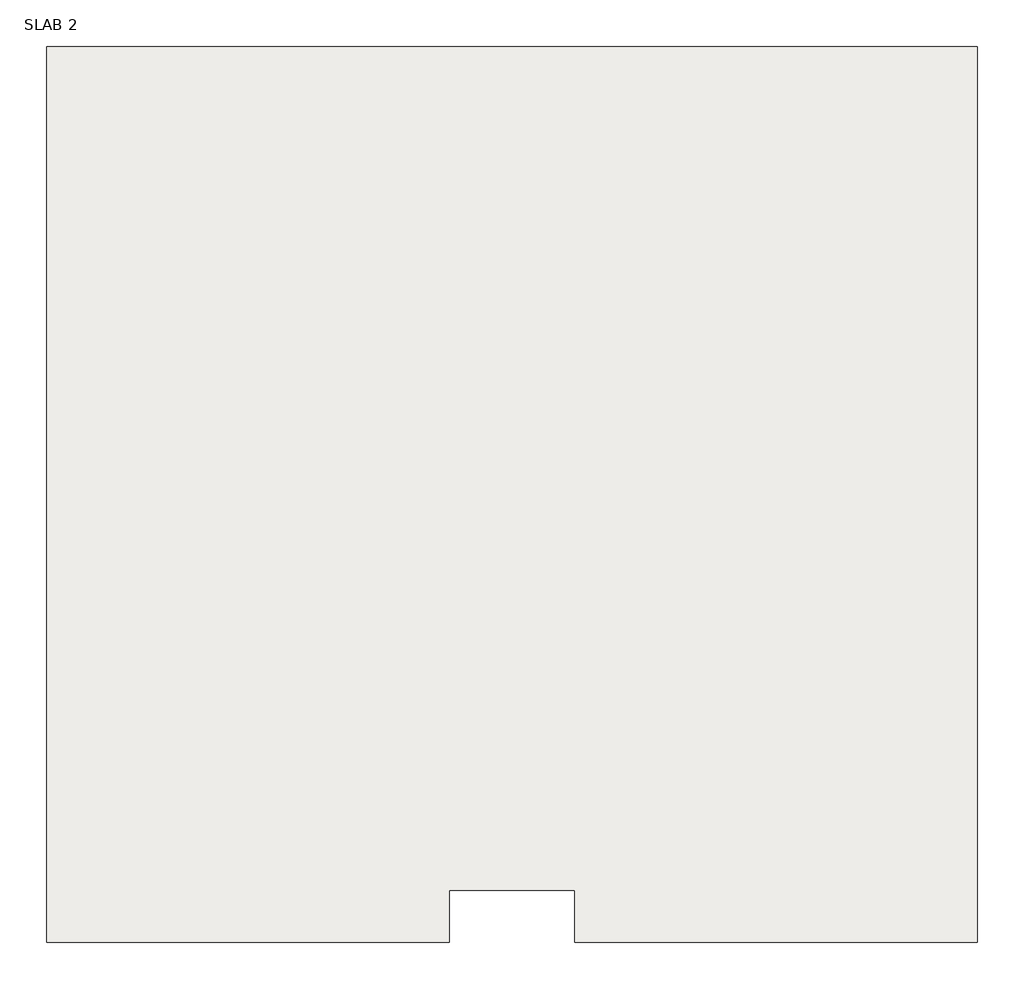
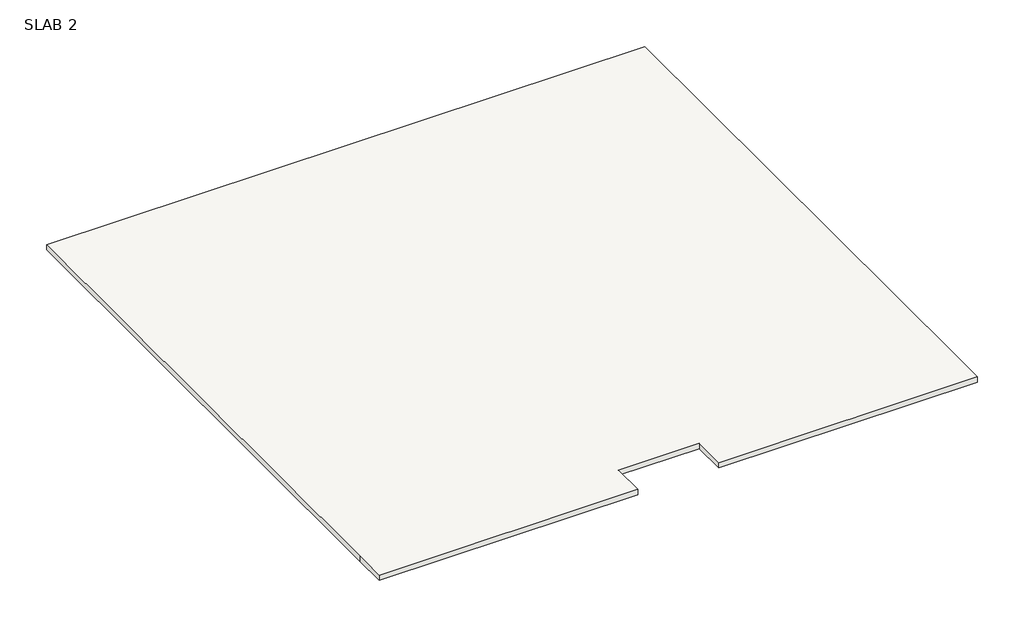
# One storey, incomplete: 1 roof.
"""IFC4 building model written with IfcOpenShell, lengths in millimetres."""

from ifc_helpers import new_model, si_unit, frame, origin, place, context, project, spatial, polyline, outline, extrude, element, save

model = new_model("IFC4")

# Units and contexts
model_context = context("Model", 3, world=origin())
ifc_project = project(units=[si_unit("LENGTHUNIT", "METRE", prefix="MILLI")], contexts=[model_context])

# Site, building, storey
site = spatial("IfcSite", under=ifc_project)
building = spatial("IfcBuilding", under=site)
storey = spatial("IfcBuildingStorey", under=building, Name="SLAB 2", Elevation=6248.4)

# Roof
placement = place(None, origin())
element("IfcRoof", 1, ObjectType="ROOFING 6\"", at=placement, inside=storey, context=model_context, shape_type="SweptSolid", body=[
    extrude(outline(polyline([(-3159.4137331, -7822.4593836), (-5369.2137331, -7822.4593836), (-5369.2137331, -8736.8593836), (-12430.4137331, -8736.8593836), (-12430.4137331, -7822.4593836), (-12430.4137331, 6987.3281164), (3901.7862669, 6987.3281164), (3901.7862669, -7822.4593836), (3901.7862669, -8736.8593836), (-3159.4137331, -8736.8593836), (-3159.4137331, -7822.4593836)])), frame((0.0, 0.0, 6248.4), z_axis=(0.0, 0.0, 1.0), x_axis=(1.0, 0.0, 0.0)), (0.0, 0.0, 1.0), 152.4),
])

save(model, "model.ifc")

# Revit data of these elements
# Type "ROOFING 6\""
#   Assembly Code = "B1020"
#   Layers, outside or top first: 0' - 6" no material (function 1)
# Element 1 (IfcRoof, "ROOFING 6\"")
#   built-in parameter 1001705 = 21 (stored number, unit not read)
#   built-in parameter 1001710 = 33615
#   Phase Created = New Construction
#   Materials on its faces: "Default Roof", "Clad - White"
# Materials
#   "Default Roof": colour RGB 88 101 114, transparency 0, Cost = 0
#   "Clad - White": class "Wood", colour RGB 242 242 238, transparency 0, Cost = 0
